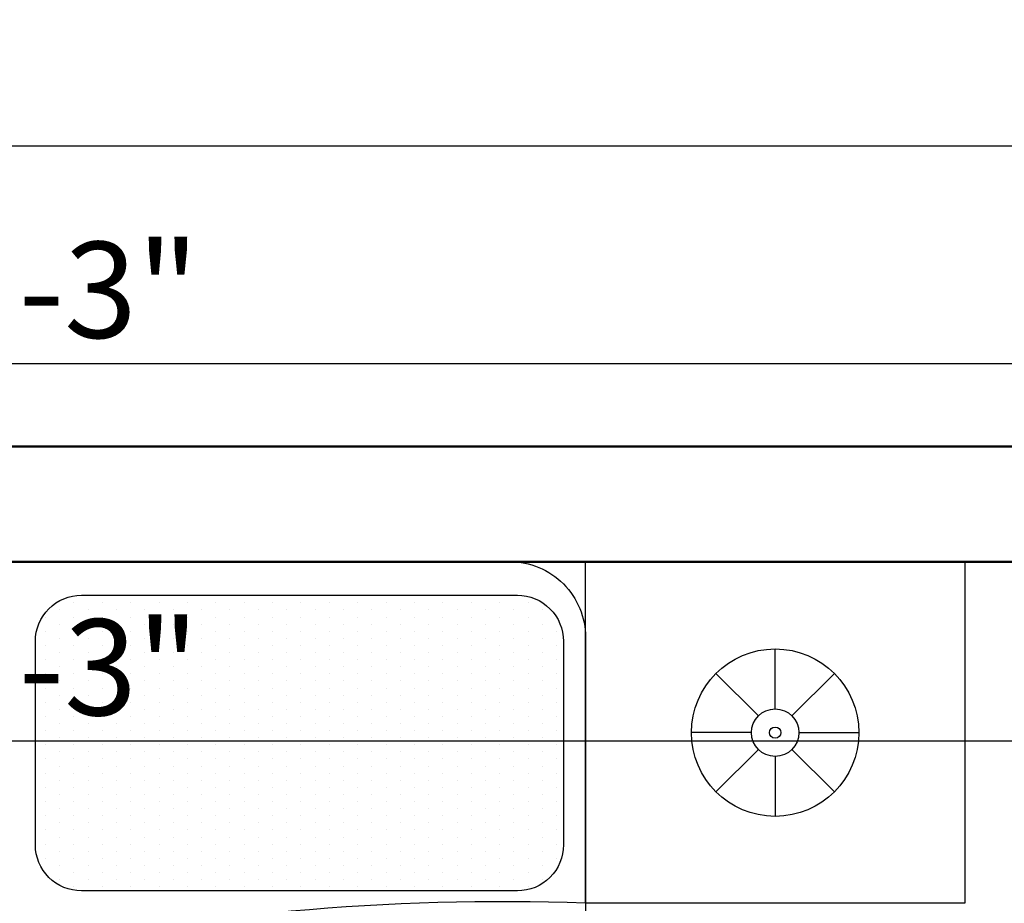
# Model space of a CAD drawing. Units: inches. Extents: x 3064 to 19385, y 846 to 15425.
# Tile 106 of 108: x 7765 to 7816, y 1373 to 1419. Entities that reach past the tile are written whole.
import ezdxf

# ---------------------------------------------------------------- set-up
doc = ezdxf.new("R2010")
doc.units = ezdxf.units.IN
for name, color, linetype, lineweight in [('A-ANNO-DIMS', 2, 'Continuous', 18), ('A-FLOR-FIXT', 9, 'Continuous', 18), ('A-WALL', 7, 'Continuous', 50)]:
    doc.layers.add(name, color=color, linetype=linetype, lineweight=lineweight)
doc.layers.add('BLOCK', color=6, linetype='Continuous')
doc.styles.get("Standard").update_dxf_attribs({"font": 'arial.ttf'})
doc.dimstyles.new('ISO-25', dxfattribs={"dimtxt": 9, "dimasz": 2.5, "dimexe": 1.25, "dimexo": 0.625, "dimtad": 1, "dimdec": 1, "dimlunit": 3, "dimtxsty": 'Standard', "dimcen": 2.5, "dimadec": 0, "dimazin": 0, "dimtfac": 1, "dimtdec": 1, "dimtmove": 0, "dimatfit": 3, "dimfxl": 1, "dimarcsym": 0})

# ---------------------------------------------------------------- blocks, each defined once
blk = doc.blocks.new('*D338')
at = {"layer": 'A-ANNO-DIMS', "color": 0, "lineweight": -2, "transparency": 16777216}
for p, q in [((7667.246, 1396.965), (7667.246, 1401.902)), ((7862.246, 1396.965), (7862.246, 1401.902)), ((7669.746, 1400.652), (7859.746, 1400.652))]:
    blk.add_line(p, q, dxfattribs=at)
at = {"layer": 'A-ANNO-DIMS', "color": 0, "transparency": 16777216}
for points in [[(7669.746, 1401.069), (7669.746, 1400.235), (7667.246, 1400.652)], [(7859.746, 1401.069), (7859.746, 1400.235), (7862.246, 1400.652)]]:
    blk.add_solid(points, dxfattribs=at)
at = {"layer": 'Defpoints', "color": 0, "transparency": 16777216}
for p in [(7862.246, 1400.652), (7667.246, 1396.34), (7862.246, 1396.34)]:
    blk.add_point(p, dxfattribs=at)
at = {"layer": 'A-ANNO-DIMS', "color": 0, "transparency": 16777216, "insert": (7764.746, 1403.832), "char_height": 5, "attachment_point": 5}
blk.add_mtext('16\'-3"', dxfattribs=at)
blk = doc.blocks.new('*D226')
at = {"layer": 'A-ANNO-DIMS', "color": 0, "lineweight": -2, "transparency": 16777216}
for p, q in [((7526.246, 1396.965), (7526.246, 1413.199)), ((7868.246, 1396.965), (7868.246, 1413.199)), ((7865.746, 1411.949), (7528.746, 1411.949))]:
    blk.add_line(p, q, dxfattribs=at)
at = {"layer": 'A-ANNO-DIMS', "color": 0, "transparency": 16777216}
for points in [[(7528.746, 1412.366), (7528.746, 1411.533), (7526.246, 1411.949)], [(7865.746, 1412.366), (7865.746, 1411.533), (7868.246, 1411.949)]]:
    blk.add_solid(points, dxfattribs=at)
at = {"layer": 'Defpoints', "color": 0, "transparency": 16777216}
for p in [(7526.246, 1411.949), (7526.246, 1396.34), (7868.246, 1396.34)]:
    blk.add_point(p, dxfattribs=at)
at = {"layer": 'A-ANNO-DIMS', "color": 0, "transparency": 16777216, "insert": (7697.246, 1415.127), "char_height": 5, "attachment_point": 5}
blk.add_mtext('28\'-6"', dxfattribs=at)
blk = doc.blocks.new('*D248')
at = {"layer": 'A-ANNO-DIMS', "color": 0, "lineweight": -2, "transparency": 16777216}
for p, q in [((7667.246, 1389.715), (7667.246, 1379.771)), ((7862.246, 1389.715), (7862.246, 1379.771)), ((7669.746, 1381.021), (7859.746, 1381.021))]:
    blk.add_line(p, q, dxfattribs=at)
at = {"layer": 'A-ANNO-DIMS', "color": 0, "transparency": 16777216}
for points in [[(7669.746, 1381.437), (7669.746, 1380.604), (7667.246, 1381.021)], [(7859.746, 1381.437), (7859.746, 1380.604), (7862.246, 1381.021)]]:
    blk.add_solid(points, dxfattribs=at)
at = {"layer": 'Defpoints', "color": 0, "transparency": 16777216}
for p in [(7667.246, 1390.34), (7862.246, 1390.34), (7862.246, 1381.021)]:
    blk.add_point(p, dxfattribs=at)
at = {"layer": 'A-ANNO-DIMS', "color": 0, "transparency": 16777216, "insert": (7764.746, 1384.2), "char_height": 5, "attachment_point": 5}
blk.add_mtext('16\'-3"', dxfattribs=at)
blk = doc.blocks.new('*X7')
at = {"color": 0}
for p, q in [((273.9375, 457.03125), (273.9375, 457.03125)), ((274.3125, 457.03125), (274.3125, 457.03125)), ((274.6875, 457.03125), (274.6875, 457.03125)), ((275.0625, 457.03125), (275.0625, 457.03125)), ((275.4375, 457.03125), (275.4375, 457.03125)), ((275.8125, 457.03125), (275.8125, 457.03125)), ((276.1875, 457.03125), (276.1875, 457.03125)), ((276.5625, 457.03125), (276.5625, 457.03125)), ((276.9375, 457.03125), (276.9375, 457.03125)), ((277.3125, 457.03125), (277.3125, 457.03125)), ((277.6875, 457.03125), (277.6875, 457.03125)), ((278.0625, 457.03125), (278.0625, 457.03125)), ((278.4375, 457.03125), (278.4375, 457.03125)), ((278.8125, 457.03125), (278.8125, 457.03125)), ((279.1875, 457.03125), (279.1875, 457.03125)), ((279.5625, 457.03125), (279.5625, 457.03125)), ((273.75, 456.9375), (273.75, 456.9375)), ((274.125, 456.9375), (274.125, 456.9375)), ((274.5, 456.9375), (274.5, 456.9375)), ((274.875, 456.9375), (274.875, 456.9375)), ((275.25, 456.9375), (275.25, 456.9375)), ((275.625, 456.9375), (275.625, 456.9375)), ((276, 456.9375), (276, 456.9375)), ((276.375, 456.9375), (276.375, 456.9375)), ((276.75, 456.9375), (276.75, 456.9375)), ((277.125, 456.9375), (277.125, 456.9375)), ((277.5, 456.9375), (277.5, 456.9375)), ((277.875, 456.9375), (277.875, 456.9375)), ((278.25, 456.9375), (278.25, 456.9375)), ((278.625, 456.9375), (278.625, 456.9375)), ((279, 456.9375), (279, 456.9375)), ((279.375, 456.9375), (279.375, 456.9375)), ((279.75, 456.9375), (279.75, 456.9375)), ((273.375, 456.75), (273.375, 456.75)), ((273.5625, 456.84375), (273.5625, 456.84375)), ((273.75, 456.75), (273.75, 456.75)), ((273.9375, 456.84375), (273.9375, 456.84375)), ((274.125, 456.75), (274.125, 456.75)), ((274.3125, 456.84375), (274.3125, 456.84375)), ((274.5, 456.75), (274.5, 456.75)), ((274.6875, 456.84375), (274.6875, 456.84375)), ((274.875, 456.75), (274.875, 456.75)), ((275.0625, 456.84375), (275.0625, 456.84375)), ((275.25, 456.75), (275.25, 456.75)), ((275.4375, 456.84375), (275.4375, 456.84375)), ((275.625, 456.75), (275.625, 456.75)), ((275.8125, 456.84375), (275.8125, 456.84375)), ((276, 456.75), (276, 456.75)), ((276.1875, 456.84375), (276.1875, 456.84375)), ((276.375, 456.75), (276.375, 456.75)), ((276.5625, 456.84375), (276.5625, 456.84375)), ((276.75, 456.75), (276.75, 456.75)), ((276.9375, 456.84375), (276.9375, 456.84375)), ((277.125, 456.75), (277.125, 456.75)), ((277.3125, 456.84375), (277.3125, 456.84375)), ((277.5, 456.75), (277.5, 456.75)), ((277.6875, 456.84375), (277.6875, 456.84375)), ((277.875, 456.75), (277.875, 456.75)), ((278.0625, 456.84375), (278.0625, 456.84375)), ((278.25, 456.75), (278.25, 456.75)), ((278.4375, 456.84375), (278.4375, 456.84375)), ((278.625, 456.75), (278.625, 456.75)), ((278.8125, 456.84375), (278.8125, 456.84375)), ((279, 456.75), (279, 456.75)), ((279.1875, 456.84375), (279.1875, 456.84375)), ((279.375, 456.75), (279.375, 456.75)), ((279.5625, 456.84375), (279.5625, 456.84375)), ((279.75, 456.75), (279.75, 456.75)), ((279.9375, 456.84375), (279.9375, 456.84375)), ((280.125, 456.75), (280.125, 456.75)), ((273.5625, 456.65625), (273.5625, 456.65625)), ((273.9375, 456.65625), (273.9375, 456.65625)), ((274.3125, 456.65625), (274.3125, 456.65625)), ((274.6875, 456.65625), (274.6875, 456.65625)), ((275.0625, 456.65625), (275.0625, 456.65625)), ((275.4375, 456.65625), (275.4375, 456.65625)), ((275.8125, 456.65625), (275.8125, 456.65625)), ((276.1875, 456.65625), (276.1875, 456.65625)), ((276.5625, 456.65625), (276.5625, 456.65625)), ((276.9375, 456.65625), (276.9375, 456.65625)), ((277.3125, 456.65625), (277.3125, 456.65625)), ((277.6875, 456.65625), (277.6875, 456.65625)), ((278.0625, 456.65625), (278.0625, 456.65625)), ((278.4375, 456.65625), (278.4375, 456.65625)), ((278.8125, 456.65625), (278.8125, 456.65625)), ((279.1875, 456.65625), (279.1875, 456.65625)), ((279.5625, 456.65625), (279.5625, 456.65625)), ((279.9375, 456.65625), (279.9375, 456.65625)), ((273.375, 456.5625), (273.375, 456.5625)), ((273.5625, 456.46875), (273.5625, 456.46875)), ((273.75, 456.5625), (273.75, 456.5625)), ((273.9375, 456.46875), (273.9375, 456.46875)), ((274.125, 456.5625), (274.125, 456.5625)), ((274.3125, 456.46875), (274.3125, 456.46875)), ((274.5, 456.5625), (274.5, 456.5625)), ((274.6875, 456.46875), (274.6875, 456.46875)), ((274.875, 456.5625), (274.875, 456.5625)), ((275.0625, 456.46875), (275.0625, 456.46875)), ((275.25, 456.5625), (275.25, 456.5625)), ((275.4375, 456.46875), (275.4375, 456.46875)), ((275.625, 456.5625), (275.625, 456.5625)), ((275.8125, 456.46875), (275.8125, 456.46875)), ((276, 456.5625), (276, 456.5625)), ((276.1875, 456.46875), (276.1875, 456.46875)), ((276.375, 456.5625), (276.375, 456.5625)), ((276.5625, 456.46875), (276.5625, 456.46875)), ((276.75, 456.5625), (276.75, 456.5625)), ((276.9375, 456.46875), (276.9375, 456.46875)), ((277.125, 456.5625), (277.125, 456.5625)), ((277.3125, 456.46875), (277.3125, 456.46875)), ((277.5, 456.5625), (277.5, 456.5625)), ((277.6875, 456.46875), (277.6875, 456.46875)), ((277.875, 456.5625), (277.875, 456.5625)), ((278.0625, 456.46875), (278.0625, 456.46875)), ((278.25, 456.5625), (278.25, 456.5625)), ((278.4375, 456.46875), (278.4375, 456.46875)), ((278.625, 456.5625), (278.625, 456.5625)), ((278.8125, 456.46875), (278.8125, 456.46875)), ((279, 456.5625), (279, 456.5625)), ((279.1875, 456.46875), (279.1875, 456.46875)), ((279.375, 456.5625), (279.375, 456.5625)), ((279.5625, 456.46875), (279.5625, 456.46875)), ((279.75, 456.5625), (279.75, 456.5625)), ((279.9375, 456.46875), (279.9375, 456.46875)), ((280.125, 456.5625), (280.125, 456.5625)), ((273.375, 456.375), (273.375, 456.375)), ((273.75, 456.375), (273.75, 456.375)), ((274.125, 456.375), (274.125, 456.375)), ((274.5, 456.375), (274.5, 456.375)), ((274.875, 456.375), (274.875, 456.375)), ((275.25, 456.375), (275.25, 456.375)), ((275.625, 456.375), (275.625, 456.375)), ((276, 456.375), (276, 456.375)), ((276.375, 456.375), (276.375, 456.375)), ((276.75, 456.375), (276.75, 456.375)), ((277.125, 456.375), (277.125, 456.375)), ((277.5, 456.375), (277.5, 456.375)), ((277.875, 456.375), (277.875, 456.375)), ((278.25, 456.375), (278.25, 456.375)), ((278.625, 456.375), (278.625, 456.375)), ((279, 456.375), (279, 456.375)), ((279.375, 456.375), (279.375, 456.375)), ((279.75, 456.375), (279.75, 456.375)), ((280.125, 456.375), (280.125, 456.375)), ((273.5625, 456.28125), (273.5625, 456.28125)), ((273.9375, 456.28125), (273.9375, 456.28125)), ((274.3125, 456.28125), (274.3125, 456.28125)), ((274.6875, 456.28125), (274.6875, 456.28125)), ((275.0625, 456.28125), (275.0625, 456.28125)), ((275.4375, 456.28125), (275.4375, 456.28125)), ((275.8125, 456.28125), (275.8125, 456.28125)), ((276.1875, 456.28125), (276.1875, 456.28125)), ((276.5625, 456.28125), (276.5625, 456.28125)), ((276.9375, 456.28125), (276.9375, 456.28125)), ((277.3125, 456.28125), (277.3125, 456.28125)), ((277.6875, 456.28125), (277.6875, 456.28125)), ((278.0625, 456.28125), (278.0625, 456.28125)), ((278.4375, 456.28125), (278.4375, 456.28125)), ((278.8125, 456.28125), (278.8125, 456.28125)), ((279.1875, 456.28125), (279.1875, 456.28125)), ((279.5625, 456.28125), (279.5625, 456.28125)), ((279.9375, 456.28125), (279.9375, 456.28125)), ((273.375, 456.1875), (273.375, 456.1875)), ((273.5625, 456.09375), (273.5625, 456.09375)), ((273.75, 456.1875), (273.75, 456.1875)), ((273.9375, 456.09375), (273.9375, 456.09375)), ((274.125, 456.1875), (274.125, 456.1875)), ((274.3125, 456.09375), (274.3125, 456.09375)), ((274.5, 456.1875), (274.5, 456.1875)), ((274.6875, 456.09375), (274.6875, 456.09375)), ((274.875, 456.1875), (274.875, 456.1875)), ((275.0625, 456.09375), (275.0625, 456.09375)), ((275.25, 456.1875), (275.25, 456.1875)), ((275.4375, 456.09375), (275.4375, 456.09375)), ((275.625, 456.1875), (275.625, 456.1875)), ((275.8125, 456.09375), (275.8125, 456.09375)), ((276, 456.1875), (276, 456.1875)), ((276.1875, 456.09375), (276.1875, 456.09375)), ((276.375, 456.1875), (276.375, 456.1875)), ((276.5625, 456.09375), (276.5625, 456.09375)), ((276.75, 456.1875), (276.75, 456.1875)), ((276.9375, 456.09375), (276.9375, 456.09375)), ((277.125, 456.1875), (277.125, 456.1875)), ((277.3125, 456.09375), (277.3125, 456.09375)), ((277.5, 456.1875), (277.5, 456.1875)), ((277.6875, 456.09375), (277.6875, 456.09375)), ((277.875, 456.1875), (277.875, 456.1875)), ((278.0625, 456.09375), (278.0625, 456.09375)), ((278.25, 456.1875), (278.25, 456.1875)), ((278.4375, 456.09375), (278.4375, 456.09375)), ((278.625, 456.1875), (278.625, 456.1875)), ((278.8125, 456.09375), (278.8125, 456.09375)), ((279, 456.1875), (279, 456.1875)), ((279.1875, 456.09375), (279.1875, 456.09375)), ((279.375, 456.1875), (279.375, 456.1875)), ((279.5625, 456.09375), (279.5625, 456.09375)), ((279.75, 456.1875), (279.75, 456.1875)), ((279.9375, 456.09375), (279.9375, 456.09375)), ((280.125, 456.1875), (280.125, 456.1875)), ((273.375, 456), (273.375, 456)), ((273.75, 456), (273.75, 456)), ((274.125, 456), (274.125, 456)), ((274.5, 456), (274.5, 456)), ((274.875, 456), (274.875, 456)), ((275.25, 456), (275.25, 456)), ((275.625, 456), (275.625, 456)), ((276, 456), (276, 456)), ((276.375, 456), (276.375, 456)), ((276.75, 456), (276.75, 456)), ((277.125, 456), (277.125, 456)), ((277.5, 456), (277.5, 456)), ((277.875, 456), (277.875, 456)), ((278.25, 456), (278.25, 456)), ((278.625, 456), (278.625, 456)), ((279, 456), (279, 456)), ((279.375, 456), (279.375, 456)), ((279.75, 456), (279.75, 456)), ((280.125, 456), (280.125, 456)), ((273.5625, 455.90625), (273.5625, 455.90625)), ((273.9375, 455.90625), (273.9375, 455.90625)), ((274.3125, 455.90625), (274.3125, 455.90625)), ((274.6875, 455.90625), (274.6875, 455.90625)), ((275.0625, 455.90625), (275.0625, 455.90625)), ((275.4375, 455.90625), (275.4375, 455.90625)), ((275.8125, 455.90625), (275.8125, 455.90625)), ((276.1875, 455.90625), (276.1875, 455.90625)), ((276.5625, 455.90625), (276.5625, 455.90625)), ((276.9375, 455.90625), (276.9375, 455.90625)), ((277.3125, 455.90625), (277.3125, 455.90625)), ((277.6875, 455.90625), (277.6875, 455.90625)), ((278.0625, 455.90625), (278.0625, 455.90625)), ((278.4375, 455.90625), (278.4375, 455.90625)), ((278.8125, 455.90625), (278.8125, 455.90625)), ((279.1875, 455.90625), (279.1875, 455.90625)), ((279.5625, 455.90625), (279.5625, 455.90625)), ((279.9375, 455.90625), (279.9375, 455.90625)), ((273.375, 455.8125), (273.375, 455.8125)), ((273.5625, 455.71875), (273.5625, 455.71875)), ((273.75, 455.8125), (273.75, 455.8125)), ((273.9375, 455.71875), (273.9375, 455.71875)), ((274.125, 455.8125), (274.125, 455.8125)), ((274.3125, 455.71875), (274.3125, 455.71875)), ((274.5, 455.8125), (274.5, 455.8125)), ((274.6875, 455.71875), (274.6875, 455.71875)), ((274.875, 455.8125), (274.875, 455.8125)), ((275.0625, 455.71875), (275.0625, 455.71875)), ((275.25, 455.8125), (275.25, 455.8125)), ((275.4375, 455.71875), (275.4375, 455.71875)), ((275.625, 455.8125), (275.625, 455.8125)), ((275.8125, 455.71875), (275.8125, 455.71875)), ((276, 455.8125), (276, 455.8125)), ((276.1875, 455.71875), (276.1875, 455.71875)), ((276.375, 455.8125), (276.375, 455.8125)), ((276.5625, 455.71875), (276.5625, 455.71875)), ((276.75, 455.8125), (276.75, 455.8125)), ((276.9375, 455.71875), (276.9375, 455.71875)), ((277.125, 455.8125), (277.125, 455.8125)), ((277.3125, 455.71875), (277.3125, 455.71875)), ((277.5, 455.8125), (277.5, 455.8125)), ((277.6875, 455.71875), (277.6875, 455.71875)), ((277.875, 455.8125), (277.875, 455.8125)), ((278.0625, 455.71875), (278.0625, 455.71875)), ((278.25, 455.8125), (278.25, 455.8125)), ((278.4375, 455.71875), (278.4375, 455.71875)), ((278.625, 455.8125), (278.625, 455.8125)), ((278.8125, 455.71875), (278.8125, 455.71875)), ((279, 455.8125), (279, 455.8125)), ((279.1875, 455.71875), (279.1875, 455.71875)), ((279.375, 455.8125), (279.375, 455.8125)), ((279.5625, 455.71875), (279.5625, 455.71875)), ((279.75, 455.8125), (279.75, 455.8125)), ((279.9375, 455.71875), (279.9375, 455.71875)), ((280.125, 455.8125), (280.125, 455.8125)), ((273.375, 455.625), (273.375, 455.625)), ((273.75, 455.625), (273.75, 455.625)), ((274.125, 455.625), (274.125, 455.625)), ((274.5, 455.625), (274.5, 455.625)), ((274.875, 455.625), (274.875, 455.625)), ((275.25, 455.625), (275.25, 455.625)), ((275.625, 455.625), (275.625, 455.625)), ((276, 455.625), (276, 455.625)), ((276.375, 455.625), (276.375, 455.625)), ((276.75, 455.625), (276.75, 455.625)), ((277.125, 455.625), (277.125, 455.625)), ((277.5, 455.625), (277.5, 455.625)), ((277.875, 455.625), (277.875, 455.625)), ((278.25, 455.625), (278.25, 455.625)), ((278.625, 455.625), (278.625, 455.625)), ((279, 455.625), (279, 455.625)), ((279.375, 455.625), (279.375, 455.625)), ((279.75, 455.625), (279.75, 455.625)), ((280.125, 455.625), (280.125, 455.625)), ((273.375, 455.4375), (273.375, 455.4375)), ((273.5625, 455.53125), (273.5625, 455.53125)), ((273.75, 455.4375), (273.75, 455.4375)), ((273.9375, 455.53125), (273.9375, 455.53125)), ((274.125, 455.4375), (274.125, 455.4375)), ((274.3125, 455.53125), (274.3125, 455.53125)), ((274.5, 455.4375), (274.5, 455.4375)), ((274.6875, 455.53125), (274.6875, 455.53125)), ((274.875, 455.4375), (274.875, 455.4375)), ((275.0625, 455.53125), (275.0625, 455.53125)), ((275.25, 455.4375), (275.25, 455.4375)), ((275.4375, 455.53125), (275.4375, 455.53125)), ((275.625, 455.4375), (275.625, 455.4375)), ((275.8125, 455.53125), (275.8125, 455.53125)), ((276, 455.4375), (276, 455.4375)), ((276.1875, 455.53125), (276.1875, 455.53125)), ((276.375, 455.4375), (276.375, 455.4375)), ((276.5625, 455.53125), (276.5625, 455.53125)), ((276.75, 455.4375), (276.75, 455.4375)), ((276.9375, 455.53125), (276.9375, 455.53125)), ((277.125, 455.4375), (277.125, 455.4375)), ((277.3125, 455.53125), (277.3125, 455.53125)), ((277.5, 455.4375), (277.5, 455.4375)), ((277.6875, 455.53125), (277.6875, 455.53125)), ((277.875, 455.4375), (277.875, 455.4375)), ((278.0625, 455.53125), (278.0625, 455.53125)), ((278.25, 455.4375), (278.25, 455.4375)), ((278.4375, 455.53125), (278.4375, 455.53125)), ((278.625, 455.4375), (278.625, 455.4375)), ((278.8125, 455.53125), (278.8125, 455.53125)), ((279, 455.4375), (279, 455.4375)), ((279.1875, 455.53125), (279.1875, 455.53125)), ((279.375, 455.4375), (279.375, 455.4375)), ((279.5625, 455.53125), (279.5625, 455.53125)), ((279.75, 455.4375), (279.75, 455.4375)), ((279.9375, 455.53125), (279.9375, 455.53125)), ((280.125, 455.4375), (280.125, 455.4375)), ((273.5625, 455.34375), (273.5625, 455.34375)), ((273.9375, 455.34375), (273.9375, 455.34375)), ((274.3125, 455.34375), (274.3125, 455.34375)), ((274.6875, 455.34375), (274.6875, 455.34375)), ((275.0625, 455.34375), (275.0625, 455.34375)), ((275.4375, 455.34375), (275.4375, 455.34375)), ((275.8125, 455.34375), (275.8125, 455.34375)), ((276.1875, 455.34375), (276.1875, 455.34375)), ((276.5625, 455.34375), (276.5625, 455.34375)), ((276.9375, 455.34375), (276.9375, 455.34375)), ((277.3125, 455.34375), (277.3125, 455.34375)), ((277.6875, 455.34375), (277.6875, 455.34375)), ((278.0625, 455.34375), (278.0625, 455.34375)), ((278.4375, 455.34375), (278.4375, 455.34375)), ((278.8125, 455.34375), (278.8125, 455.34375)), ((279.1875, 455.34375), (279.1875, 455.34375)), ((279.5625, 455.34375), (279.5625, 455.34375)), ((279.9375, 455.34375), (279.9375, 455.34375)), ((273.375, 455.25), (273.375, 455.25)), ((273.75, 455.25), (273.75, 455.25)), ((274.125, 455.25), (274.125, 455.25)), ((274.5, 455.25), (274.5, 455.25)), ((274.875, 455.25), (274.875, 455.25)), ((275.25, 455.25), (275.25, 455.25)), ((275.625, 455.25), (275.625, 455.25)), ((276, 455.25), (276, 455.25)), ((276.375, 455.25), (276.375, 455.25)), ((276.75, 455.25), (276.75, 455.25)), ((277.125, 455.25), (277.125, 455.25)), ((277.5, 455.25), (277.5, 455.25)), ((277.875, 455.25), (277.875, 455.25)), ((278.25, 455.25), (278.25, 455.25)), ((278.625, 455.25), (278.625, 455.25)), ((279, 455.25), (279, 455.25)), ((279.375, 455.25), (279.375, 455.25)), ((279.75, 455.25), (279.75, 455.25)), ((280.125, 455.25), (280.125, 455.25)), ((273.375, 455.0625), (273.375, 455.0625)), ((273.5625, 455.15625), (273.5625, 455.15625)), ((273.75, 455.0625), (273.75, 455.0625)), ((273.9375, 455.15625), (273.9375, 455.15625)), ((274.125, 455.0625), (274.125, 455.0625)), ((274.3125, 455.15625), (274.3125, 455.15625)), ((274.5, 455.0625), (274.5, 455.0625)), ((274.6875, 455.15625), (274.6875, 455.15625)), ((274.875, 455.0625), (274.875, 455.0625)), ((275.0625, 455.15625), (275.0625, 455.15625)), ((275.25, 455.0625), (275.25, 455.0625)), ((275.4375, 455.15625), (275.4375, 455.15625)), ((275.625, 455.0625), (275.625, 455.0625)), ((275.8125, 455.15625), (275.8125, 455.15625)), ((276, 455.0625), (276, 455.0625)), ((276.1875, 455.15625), (276.1875, 455.15625)), ((276.375, 455.0625), (276.375, 455.0625)), ((276.5625, 455.15625), (276.5625, 455.15625)), ((276.75, 455.0625), (276.75, 455.0625)), ((276.9375, 455.15625), (276.9375, 455.15625)), ((277.125, 455.0625), (277.125, 455.0625)), ((277.3125, 455.15625), (277.3125, 455.15625)), ((277.5, 455.0625), (277.5, 455.0625)), ((277.6875, 455.15625), (277.6875, 455.15625)), ((277.875, 455.0625), (277.875, 455.0625)), ((278.0625, 455.15625), (278.0625, 455.15625)), ((278.25, 455.0625), (278.25, 455.0625)), ((278.4375, 455.15625), (278.4375, 455.15625)), ((278.625, 455.0625), (278.625, 455.0625)), ((278.8125, 455.15625), (278.8125, 455.15625)), ((279, 455.0625), (279, 455.0625)), ((279.1875, 455.15625), (279.1875, 455.15625)), ((279.375, 455.0625), (279.375, 455.0625)), ((279.5625, 455.15625), (279.5625, 455.15625)), ((279.75, 455.0625), (279.75, 455.0625)), ((279.9375, 455.15625), (279.9375, 455.15625)), ((280.125, 455.0625), (280.125, 455.0625)), ((273.5625, 454.96875), (273.5625, 454.96875)), ((273.9375, 454.96875), (273.9375, 454.96875)), ((274.3125, 454.96875), (274.3125, 454.96875)), ((274.6875, 454.96875), (274.6875, 454.96875)), ((275.0625, 454.96875), (275.0625, 454.96875)), ((275.4375, 454.96875), (275.4375, 454.96875)), ((275.8125, 454.96875), (275.8125, 454.96875)), ((276.1875, 454.96875), (276.1875, 454.96875)), ((276.5625, 454.96875), (276.5625, 454.96875)), ((276.9375, 454.96875), (276.9375, 454.96875)), ((277.3125, 454.96875), (277.3125, 454.96875)), ((277.6875, 454.96875), (277.6875, 454.96875)), ((278.0625, 454.96875), (278.0625, 454.96875)), ((278.4375, 454.96875), (278.4375, 454.96875)), ((278.8125, 454.96875), (278.8125, 454.96875)), ((279.1875, 454.96875), (279.1875, 454.96875)), ((279.5625, 454.96875), (279.5625, 454.96875)), ((279.9375, 454.96875), (279.9375, 454.96875)), ((273.375, 454.875), (273.375, 454.875)), ((273.5625, 454.78125), (273.5625, 454.78125)), ((273.75, 454.875), (273.75, 454.875)), ((273.9375, 454.78125), (273.9375, 454.78125)), ((274.125, 454.875), (274.125, 454.875)), ((274.3125, 454.78125), (274.3125, 454.78125)), ((274.5, 454.875), (274.5, 454.875)), ((274.6875, 454.78125), (274.6875, 454.78125)), ((274.875, 454.875), (274.875, 454.875)), ((275.0625, 454.78125), (275.0625, 454.78125)), ((275.25, 454.875), (275.25, 454.875)), ((275.4375, 454.78125), (275.4375, 454.78125)), ((275.625, 454.875), (275.625, 454.875)), ((275.8125, 454.78125), (275.8125, 454.78125)), ((276, 454.875), (276, 454.875)), ((276.1875, 454.78125), (276.1875, 454.78125)), ((276.375, 454.875), (276.375, 454.875)), ((276.5625, 454.78125), (276.5625, 454.78125)), ((276.75, 454.875), (276.75, 454.875)), ((276.9375, 454.78125), (276.9375, 454.78125)), ((277.125, 454.875), (277.125, 454.875)), ((277.3125, 454.78125), (277.3125, 454.78125)), ((277.5, 454.875), (277.5, 454.875)), ((277.6875, 454.78125), (277.6875, 454.78125)), ((277.875, 454.875), (277.875, 454.875)), ((278.0625, 454.78125), (278.0625, 454.78125)), ((278.25, 454.875), (278.25, 454.875)), ((278.4375, 454.78125), (278.4375, 454.78125)), ((278.625, 454.875), (278.625, 454.875)), ((278.8125, 454.78125), (278.8125, 454.78125)), ((279, 454.875), (279, 454.875)), ((279.1875, 454.78125), (279.1875, 454.78125)), ((279.375, 454.875), (279.375, 454.875)), ((279.5625, 454.78125), (279.5625, 454.78125)), ((279.75, 454.875), (279.75, 454.875)), ((279.9375, 454.78125), (279.9375, 454.78125)), ((280.125, 454.875), (280.125, 454.875)), ((273.375, 454.6875), (273.375, 454.6875)), ((273.75, 454.6875), (273.75, 454.6875)), ((274.125, 454.6875), (274.125, 454.6875)), ((274.5, 454.6875), (274.5, 454.6875)), ((274.875, 454.6875), (274.875, 454.6875)), ((275.25, 454.6875), (275.25, 454.6875)), ((275.625, 454.6875), (275.625, 454.6875)), ((276, 454.6875), (276, 454.6875)), ((276.375, 454.6875), (276.375, 454.6875)), ((276.75, 454.6875), (276.75, 454.6875)), ((277.125, 454.6875), (277.125, 454.6875)), ((277.5, 454.6875), (277.5, 454.6875)), ((277.875, 454.6875), (277.875, 454.6875)), ((278.25, 454.6875), (278.25, 454.6875)), ((278.625, 454.6875), (278.625, 454.6875)), ((279, 454.6875), (279, 454.6875)), ((279.375, 454.6875), (279.375, 454.6875)), ((279.75, 454.6875), (279.75, 454.6875)), ((280.125, 454.6875), (280.125, 454.6875)), ((273.5625, 454.59375), (273.5625, 454.59375)), ((273.9375, 454.59375), (273.9375, 454.59375)), ((274.3125, 454.59375), (274.3125, 454.59375)), ((274.6875, 454.59375), (274.6875, 454.59375)), ((275.0625, 454.59375), (275.0625, 454.59375)), ((275.4375, 454.59375), (275.4375, 454.59375)), ((275.8125, 454.59375), (275.8125, 454.59375)), ((276.1875, 454.59375), (276.1875, 454.59375)), ((276.5625, 454.59375), (276.5625, 454.59375)), ((276.9375, 454.59375), (276.9375, 454.59375)), ((277.3125, 454.59375), (277.3125, 454.59375)), ((277.6875, 454.59375), (277.6875, 454.59375)), ((278.0625, 454.59375), (278.0625, 454.59375)), ((278.4375, 454.59375), (278.4375, 454.59375)), ((278.8125, 454.59375), (278.8125, 454.59375)), ((279.1875, 454.59375), (279.1875, 454.59375)), ((279.5625, 454.59375), (279.5625, 454.59375)), ((279.9375, 454.59375), (279.9375, 454.59375)), ((273.375, 454.5), (273.375, 454.5)), ((273.5625, 454.40625), (273.5625, 454.40625)), ((273.75, 454.5), (273.75, 454.5)), ((273.9375, 454.40625), (273.9375, 454.40625)), ((274.125, 454.5), (274.125, 454.5)), ((274.3125, 454.40625), (274.3125, 454.40625)), ((274.5, 454.5), (274.5, 454.5)), ((274.6875, 454.40625), (274.6875, 454.40625)), ((274.875, 454.5), (274.875, 454.5)), ((275.0625, 454.40625), (275.0625, 454.40625)), ((275.25, 454.5), (275.25, 454.5)), ((275.4375, 454.40625), (275.4375, 454.40625)), ((275.625, 454.5), (275.625, 454.5)), ((275.8125, 454.40625), (275.8125, 454.40625)), ((276, 454.5), (276, 454.5)), ((276.1875, 454.40625), (276.1875, 454.40625)), ((276.375, 454.5), (276.375, 454.5)), ((276.5625, 454.40625), (276.5625, 454.40625)), ((276.75, 454.5), (276.75, 454.5)), ((276.9375, 454.40625), (276.9375, 454.40625)), ((277.125, 454.5), (277.125, 454.5)), ((277.3125, 454.40625), (277.3125, 454.40625)), ((277.5, 454.5), (277.5, 454.5)), ((277.6875, 454.40625), (277.6875, 454.40625)), ((277.875, 454.5), (277.875, 454.5)), ((278.0625, 454.40625), (278.0625, 454.40625)), ((278.25, 454.5), (278.25, 454.5)), ((278.4375, 454.40625), (278.4375, 454.40625)), ((278.625, 454.5), (278.625, 454.5)), ((278.8125, 454.40625), (278.8125, 454.40625)), ((279, 454.5), (279, 454.5)), ((279.1875, 454.40625), (279.1875, 454.40625)), ((279.375, 454.5), (279.375, 454.5)), ((279.5625, 454.40625), (279.5625, 454.40625)), ((279.75, 454.5), (279.75, 454.5)), ((279.9375, 454.40625), (279.9375, 454.40625)), ((280.125, 454.5), (280.125, 454.5)), ((273.375, 454.3125), (273.375, 454.3125)), ((273.75, 454.3125), (273.75, 454.3125)), ((274.125, 454.3125), (274.125, 454.3125)), ((274.5, 454.3125), (274.5, 454.3125)), ((274.875, 454.3125), (274.875, 454.3125)), ((275.25, 454.3125), (275.25, 454.3125)), ((275.625, 454.3125), (275.625, 454.3125)), ((276, 454.3125), (276, 454.3125)), ((276.375, 454.3125), (276.375, 454.3125)), ((276.75, 454.3125), (276.75, 454.3125)), ((277.125, 454.3125), (277.125, 454.3125)), ((277.5, 454.3125), (277.5, 454.3125)), ((277.875, 454.3125), (277.875, 454.3125)), ((278.25, 454.3125), (278.25, 454.3125)), ((278.625, 454.3125), (278.625, 454.3125)), ((279, 454.3125), (279, 454.3125)), ((279.375, 454.3125), (279.375, 454.3125)), ((279.75, 454.3125), (279.75, 454.3125)), ((280.125, 454.3125), (280.125, 454.3125)), ((273.375, 454.125), (273.375, 454.125)), ((273.5625, 454.21875), (273.5625, 454.21875)), ((273.75, 454.125), (273.75, 454.125)), ((273.9375, 454.21875), (273.9375, 454.21875)), ((274.125, 454.125), (274.125, 454.125)), ((274.3125, 454.21875), (274.3125, 454.21875)), ((274.5, 454.125), (274.5, 454.125)), ((274.6875, 454.21875), (274.6875, 454.21875)), ((274.875, 454.125), (274.875, 454.125)), ((275.0625, 454.21875), (275.0625, 454.21875)), ((275.25, 454.125), (275.25, 454.125)), ((275.4375, 454.21875), (275.4375, 454.21875)), ((275.625, 454.125), (275.625, 454.125)), ((275.8125, 454.21875), (275.8125, 454.21875)), ((276, 454.125), (276, 454.125)), ((276.1875, 454.21875), (276.1875, 454.21875)), ((276.375, 454.125), (276.375, 454.125)), ((276.5625, 454.21875), (276.5625, 454.21875)), ((276.75, 454.125), (276.75, 454.125)), ((276.9375, 454.21875), (276.9375, 454.21875)), ((277.125, 454.125), (277.125, 454.125)), ((277.3125, 454.21875), (277.3125, 454.21875)), ((277.5, 454.125), (277.5, 454.125)), ((277.6875, 454.21875), (277.6875, 454.21875)), ((277.875, 454.125), (277.875, 454.125)), ((278.0625, 454.21875), (278.0625, 454.21875)), ((278.25, 454.125), (278.25, 454.125)), ((278.4375, 454.21875), (278.4375, 454.21875)), ((278.625, 454.125), (278.625, 454.125)), ((278.8125, 454.21875), (278.8125, 454.21875)), ((279, 454.125), (279, 454.125)), ((279.1875, 454.21875), (279.1875, 454.21875)), ((279.375, 454.125), (279.375, 454.125)), ((279.5625, 454.21875), (279.5625, 454.21875)), ((279.75, 454.125), (279.75, 454.125)), ((279.9375, 454.21875), (279.9375, 454.21875)), ((280.125, 454.125), (280.125, 454.125)), ((273.5625, 454.03125), (273.5625, 454.03125)), ((273.9375, 454.03125), (273.9375, 454.03125)), ((274.3125, 454.03125), (274.3125, 454.03125)), ((274.6875, 454.03125), (274.6875, 454.03125)), ((275.0625, 454.03125), (275.0625, 454.03125)), ((275.4375, 454.03125), (275.4375, 454.03125)), ((275.8125, 454.03125), (275.8125, 454.03125)), ((276.1875, 454.03125), (276.1875, 454.03125)), ((276.5625, 454.03125), (276.5625, 454.03125)), ((276.9375, 454.03125), (276.9375, 454.03125)), ((277.3125, 454.03125), (277.3125, 454.03125)), ((277.6875, 454.03125), (277.6875, 454.03125)), ((278.0625, 454.03125), (278.0625, 454.03125)), ((278.4375, 454.03125), (278.4375, 454.03125)), ((278.8125, 454.03125), (278.8125, 454.03125)), ((279.1875, 454.03125), (279.1875, 454.03125)), ((279.5625, 454.03125), (279.5625, 454.03125)), ((279.9375, 454.03125), (279.9375, 454.03125)), ((273.375, 453.9375), (273.375, 453.9375)), ((273.75, 453.9375), (273.75, 453.9375)), ((274.125, 453.9375), (274.125, 453.9375)), ((274.5, 453.9375), (274.5, 453.9375)), ((274.875, 453.9375), (274.875, 453.9375)), ((275.25, 453.9375), (275.25, 453.9375)), ((275.625, 453.9375), (275.625, 453.9375)), ((276, 453.9375), (276, 453.9375)), ((276.375, 453.9375), (276.375, 453.9375)), ((276.75, 453.9375), (276.75, 453.9375)), ((277.125, 453.9375), (277.125, 453.9375)), ((277.5, 453.9375), (277.5, 453.9375)), ((277.875, 453.9375), (277.875, 453.9375)), ((278.25, 453.9375), (278.25, 453.9375)), ((278.625, 453.9375), (278.625, 453.9375)), ((279, 453.9375), (279, 453.9375)), ((279.375, 453.9375), (279.375, 453.9375)), ((279.75, 453.9375), (279.75, 453.9375)), ((280.125, 453.9375), (280.125, 453.9375)), ((273.375, 453.75), (273.375, 453.75)), ((273.5625, 453.84375), (273.5625, 453.84375)), ((273.75, 453.75), (273.75, 453.75)), ((273.9375, 453.84375), (273.9375, 453.84375)), ((274.125, 453.75), (274.125, 453.75)), ((274.3125, 453.84375), (274.3125, 453.84375)), ((274.5, 453.75), (274.5, 453.75)), ((274.6875, 453.84375), (274.6875, 453.84375)), ((274.875, 453.75), (274.875, 453.75)), ((275.0625, 453.84375), (275.0625, 453.84375)), ((275.25, 453.75), (275.25, 453.75)), ((275.4375, 453.84375), (275.4375, 453.84375)), ((275.625, 453.75), (275.625, 453.75)), ((275.8125, 453.84375), (275.8125, 453.84375)), ((276, 453.75), (276, 453.75)), ((276.1875, 453.84375), (276.1875, 453.84375)), ((276.375, 453.75), (276.375, 453.75)), ((276.5625, 453.84375), (276.5625, 453.84375)), ((276.75, 453.75), (276.75, 453.75)), ((276.9375, 453.84375), (276.9375, 453.84375)), ((277.125, 453.75), (277.125, 453.75)), ((277.3125, 453.84375), (277.3125, 453.84375)), ((277.5, 453.75), (277.5, 453.75)), ((277.6875, 453.84375), (277.6875, 453.84375)), ((277.875, 453.75), (277.875, 453.75)), ((278.0625, 453.84375), (278.0625, 453.84375)), ((278.25, 453.75), (278.25, 453.75)), ((278.4375, 453.84375), (278.4375, 453.84375)), ((278.625, 453.75), (278.625, 453.75)), ((278.8125, 453.84375), (278.8125, 453.84375)), ((279, 453.75), (279, 453.75)), ((279.1875, 453.84375), (279.1875, 453.84375)), ((279.375, 453.75), (279.375, 453.75)), ((279.5625, 453.84375), (279.5625, 453.84375)), ((279.75, 453.75), (279.75, 453.75)), ((279.9375, 453.84375), (279.9375, 453.84375)), ((280.125, 453.75), (280.125, 453.75)), ((273.5625, 453.65625), (273.5625, 453.65625)), ((273.9375, 453.65625), (273.9375, 453.65625)), ((274.3125, 453.65625), (274.3125, 453.65625)), ((274.6875, 453.65625), (274.6875, 453.65625)), ((275.0625, 453.65625), (275.0625, 453.65625)), ((275.4375, 453.65625), (275.4375, 453.65625)), ((275.8125, 453.65625), (275.8125, 453.65625)), ((276.1875, 453.65625), (276.1875, 453.65625)), ((276.5625, 453.65625), (276.5625, 453.65625)), ((276.9375, 453.65625), (276.9375, 453.65625)), ((277.3125, 453.65625), (277.3125, 453.65625)), ((277.6875, 453.65625), (277.6875, 453.65625)), ((278.0625, 453.65625), (278.0625, 453.65625)), ((278.4375, 453.65625), (278.4375, 453.65625)), ((278.8125, 453.65625), (278.8125, 453.65625)), ((279.1875, 453.65625), (279.1875, 453.65625)), ((279.5625, 453.65625), (279.5625, 453.65625)), ((279.9375, 453.65625), (279.9375, 453.65625)), ((273.375, 453.5625), (273.375, 453.5625)), ((273.75, 453.5625), (273.75, 453.5625)), ((274.125, 453.5625), (274.125, 453.5625)), ((274.5, 453.5625), (274.5, 453.5625)), ((274.875, 453.5625), (274.875, 453.5625)), ((275.25, 453.5625), (275.25, 453.5625)), ((275.625, 453.5625), (275.625, 453.5625)), ((276, 453.5625), (276, 453.5625)), ((276.375, 453.5625), (276.375, 453.5625)), ((276.75, 453.5625), (276.75, 453.5625)), ((277.125, 453.5625), (277.125, 453.5625)), ((277.5, 453.5625), (277.5, 453.5625)), ((277.875, 453.5625), (277.875, 453.5625)), ((278.25, 453.5625), (278.25, 453.5625)), ((278.625, 453.5625), (278.625, 453.5625)), ((279, 453.5625), (279, 453.5625)), ((279.375, 453.5625), (279.375, 453.5625)), ((279.75, 453.5625), (279.75, 453.5625)), ((280.125, 453.5625), (280.125, 453.5625)), ((273.375, 453.375), (273.375, 453.375)), ((273.5625, 453.46875), (273.5625, 453.46875)), ((273.75, 453.375), (273.75, 453.375)), ((273.9375, 453.46875), (273.9375, 453.46875)), ((274.125, 453.375), (274.125, 453.375)), ((274.3125, 453.46875), (274.3125, 453.46875)), ((274.5, 453.375), (274.5, 453.375)), ((274.6875, 453.46875), (274.6875, 453.46875)), ((274.875, 453.375), (274.875, 453.375)), ((275.0625, 453.46875), (275.0625, 453.46875)), ((275.25, 453.375), (275.25, 453.375)), ((275.4375, 453.46875), (275.4375, 453.46875)), ((275.625, 453.375), (275.625, 453.375)), ((275.8125, 453.46875), (275.8125, 453.46875)), ((276, 453.375), (276, 453.375)), ((276.1875, 453.46875), (276.1875, 453.46875)), ((276.375, 453.375), (276.375, 453.375)), ((276.5625, 453.46875), (276.5625, 453.46875)), ((276.75, 453.375), (276.75, 453.375)), ((276.9375, 453.46875), (276.9375, 453.46875)), ((277.125, 453.375), (277.125, 453.375)), ((277.3125, 453.46875), (277.3125, 453.46875)), ((277.5, 453.375), (277.5, 453.375)), ((277.6875, 453.46875), (277.6875, 453.46875)), ((277.875, 453.375), (277.875, 453.375)), ((278.0625, 453.46875), (278.0625, 453.46875)), ((278.25, 453.375), (278.25, 453.375)), ((278.4375, 453.46875), (278.4375, 453.46875)), ((278.625, 453.375), (278.625, 453.375)), ((278.8125, 453.46875), (278.8125, 453.46875)), ((279, 453.375), (279, 453.375)), ((279.1875, 453.46875), (279.1875, 453.46875)), ((279.375, 453.375), (279.375, 453.375)), ((279.5625, 453.46875), (279.5625, 453.46875)), ((279.75, 453.375), (279.75, 453.375)), ((279.9375, 453.46875), (279.9375, 453.46875)), ((273.5625, 453.28125), (273.5625, 453.28125)), ((273.9375, 453.28125), (273.9375, 453.28125)), ((274.3125, 453.28125), (274.3125, 453.28125)), ((274.6875, 453.28125), (274.6875, 453.28125)), ((275.0625, 453.28125), (275.0625, 453.28125)), ((275.4375, 453.28125), (275.4375, 453.28125)), ((275.8125, 453.28125), (275.8125, 453.28125)), ((276.1875, 453.28125), (276.1875, 453.28125)), ((276.5625, 453.28125), (276.5625, 453.28125)), ((276.9375, 453.28125), (276.9375, 453.28125)), ((277.3125, 453.28125), (277.3125, 453.28125)), ((277.6875, 453.28125), (277.6875, 453.28125)), ((278.0625, 453.28125), (278.0625, 453.28125)), ((278.4375, 453.28125), (278.4375, 453.28125)), ((278.8125, 453.28125), (278.8125, 453.28125)), ((279.1875, 453.28125), (279.1875, 453.28125)), ((279.5625, 453.28125), (279.5625, 453.28125)), ((279.9375, 453.28125), (279.9375, 453.28125)), ((273.75, 453.1875), (273.75, 453.1875)), ((274.125, 453.1875), (274.125, 453.1875)), ((274.5, 453.1875), (274.5, 453.1875)), ((274.875, 453.1875), (274.875, 453.1875)), ((275.25, 453.1875), (275.25, 453.1875)), ((275.625, 453.1875), (275.625, 453.1875)), ((276, 453.1875), (276, 453.1875)), ((276.375, 453.1875), (276.375, 453.1875)), ((276.75, 453.1875), (276.75, 453.1875)), ((277.125, 453.1875), (277.125, 453.1875)), ((277.5, 453.1875), (277.5, 453.1875)), ((277.875, 453.1875), (277.875, 453.1875)), ((278.25, 453.1875), (278.25, 453.1875)), ((278.625, 453.1875), (278.625, 453.1875)), ((279, 453.1875), (279, 453.1875)), ((279.375, 453.1875), (279.375, 453.1875)), ((279.75, 453.1875), (279.75, 453.1875))]:
    blk.add_line(p, q, dxfattribs=at)
blk = doc.blocks.new('A$C52E67D0D')
at = {"layer": 'BLOCK'}
for p, q in [((2251.5, 1605.5), (2251.5, 1684.7)), ((2229.3, 1596.3), (2173.3, 1652.3)), ((2273.7, 1596.3), (2329.7, 1652.3)), ((2220.1, 1574.1), (2140.9, 1574.1)), ((2282.9, 1574.1), (2362.1, 1574.1)), ((2229.3, 1551.9), (2173.3, 1495.9)), ((2273.7, 1551.9), (2329.7, 1495.9)), ((2251.5, 1542.8), (2251.5, 1463.5))]:
    blk.add_line(p, q, dxfattribs=at)
for points in [[(1901, 0), (601, 0, -0.414214), (501, 100), (501, 1700, -0.414214), (601, 1800), (1901, 1800, -0.414214), (2001, 1700), (2001, 100, -0.414214)], [(1911, 1365.1), (1335, 1365.1, -0.414214), (1274.2, 1425.9), (1274.2, 1694.8, -0.414214), (1335, 1755.7), (1911, 1755.7, -0.414214), (1971.8, 1694.8), (1971.8, 1425.9, -0.414214)]]:
    blk.add_lwpolyline(points, format="xyb", close=True, dxfattribs=at)
blk.add_lwpolyline([(2001, 1348.6), (2001, 1799.6), (2502, 1799.6), (2502, 1348.6)], close=True, dxfattribs=at)
for radius in [110.6, 31.4, 7.46]:
    blk.add_circle((2251.5, 1574.1), radius, dxfattribs=at)
blk.add_arc((1888.6, -1664.5), 3015.3, 87.8642, 117.4001, dxfattribs=at)
at = {"layer": 'BLOCK', "xscale": 100, "yscale": 100, "zscale": 100}
blk.add_blockref('*X7', (-26050, -43948.2), dxfattribs=at)

msp = doc.modelspace()

# ---------------------------------------------------------------- linework, layer by layer
at = {"layer": 'A-WALL'}
for p, q in [((7868.246, 1396.34), (7526.246, 1396.34)), ((7862.246, 1390.34), (7667.246, 1390.34))]:
    msp.add_line(p, q, dxfattribs=at)

# ---------------------------------------------------------------- block references
at = {"layer": 'A-FLOR-FIXT', "xscale": 0.039370099999992, "yscale": 0.039370099999992, "zscale": 0.039370099999992}
msp.add_blockref('A$C52E67D0D', (7715.494, 1319.474), dxfattribs=at)

# ---------------------------------------------------------------- dimensions: what is measured, and where the dimension line sits
at = {"layer": 'A-ANNO-DIMS'}
for base, p1, p2, override, picture, middle in [((7526.246, 1411.949), (7868.246, 1396.34), (7526.246, 1396.34), {"dimtxt": 5, "dimclrd": 0, "dimclre": 0, "dimclrt": 0}, '*D226', (7697.246, 1415.127)), ((7862.246, 1400.652), (7667.246, 1396.34), (7862.246, 1396.34), {"dimtxt": 5, "dimclrd": 0, "dimclre": 0, "dimclrt": 0, "dimtmove": 1}, '*D338', (7764.746, 1403.832)), ((7862.246, 1381.021), (7667.246, 1390.34), (7862.246, 1390.34), {"dimtxt": 5, "dimclrd": 0, "dimclre": 0, "dimclrt": 0}, '*D248', (7764.746, 1384.2))]:
    dim = msp.add_linear_dim(base=base, p1=p1, p2=p2, dimstyle='ISO-25', override=override, dxfattribs=at)
    dim.commit()
    dim.dimension.update_dxf_attribs({"geometry": picture, "text_midpoint": middle})

doc.saveas('drawing.dxf')
